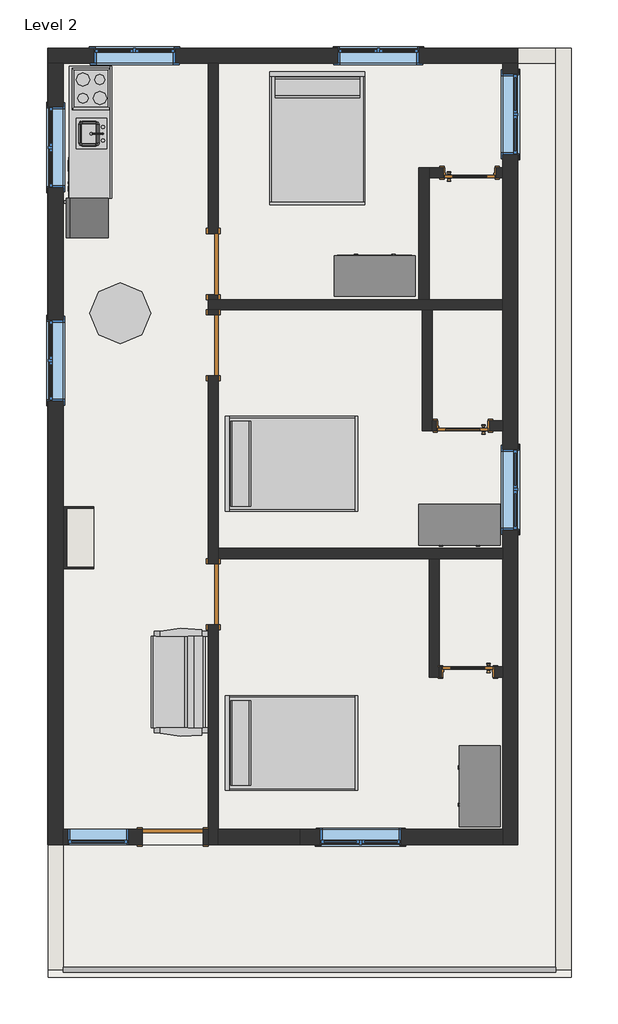
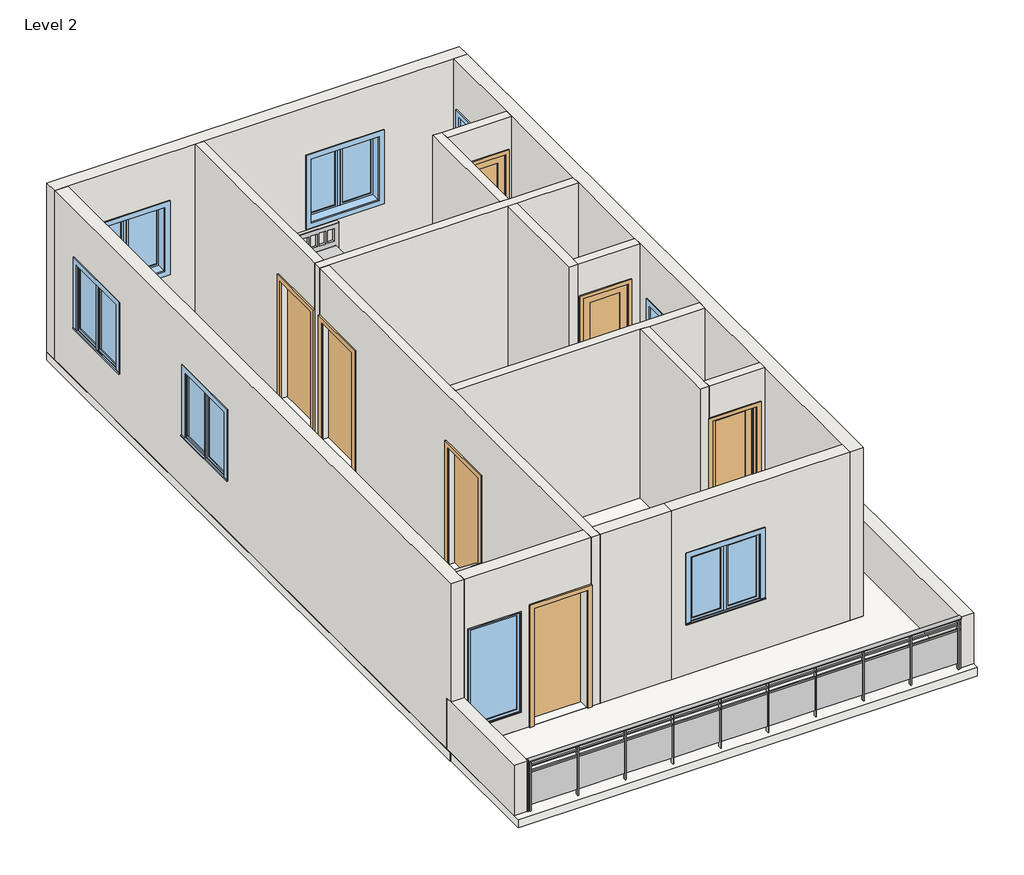
# One storey, incomplete: 20 walls, 9 furniture elements, 8 windows, 7 doors, 4 proxies, 2 slabs, 1 flow terminal, 1 railing.
"""IFC4 building model written with IfcOpenShell, lengths in millimetres."""

from ifc_helpers import new_model, si_unit, point, frame, origin, place, context, project, spatial, polyline, ellipse_curve, trimmed, outline, extrude, faceted_brep, transform, mapped, element, save
from ifc_brep_helpers import plane_surface, extruded_surface, advanced_brep
from components import proxy_a6faaae8, proxy_45b28599, kitchenette_medium_kitchenette_medium_844211aa, proxy_c523a7b7, m_door_interior_single_1_panel_wood_750_x_2400mm_65023cff, m_door_interior_single_1_panel_wood_750_x_2400mm_f8366a1a, door_16372e1c, door_686f89d2, door_0ca8825f, flow_terminal_871c2e40, furniture_096e7f55, furniture_c6510c7c, m_dresser_1220_x_1830_x_0610mm_7cb11019, m_sofa_pensi_2134mm_8f487940, furniture_905aceb5, walls_2_walls_1_3d7729ba, window_534dcd48, window_c796fc87

model = new_model("IFC4")

# Units and contexts
model_context = context("Model", 3, world=origin())
ifc_project = project(units=[si_unit("LENGTHUNIT", "METRE", prefix="MILLI")], contexts=[model_context])

# Site, building, storey
site = spatial("IfcSite", under=ifc_project)
building = spatial("IfcBuilding", under=site)
storey = spatial("IfcBuildingStorey", under=building, Name="Level 2", Elevation=3200.4)

# Proxies
placement = place(None, origin())
proxy_shape = proxy_a6faaae8(model_context)
element("IfcBuildingElementProxy", 1, Name="Cook Top-4 Unit2 : 22\" x 20\"", ObjectType="Cook Top-4 Unit2 : 22\" x 20\"", at=placement, inside=storey, context=model_context, shape_type="MappedRepresentation", body=[
    mapped(proxy_shape, transform((-8891.8371236, 5030.6122215, 3200.4), x_axis=(0.0, -1.0000000000000002, 0.0), y_axis=(1.0000000000000002, 0.0, 0.0), z_axis=(0.0, 0.0, 1.0))),
])
proxy_2_shape = proxy_45b28599(model_context)
element("IfcBuildingElementProxy", 2, Name="Dishwasher : 24\" x 24\" x 34\"", ObjectType="Dishwasher : 24\" x 24\" x 34\"", at=placement, inside=storey, context=model_context, shape_type="MappedRepresentation", body=[
    mapped(proxy_2_shape, transform((-9183.6866883, 4079.42969, 3200.4), x_axis=(0.0, -1.0000000000000002, 0.0), y_axis=(1.0000000000000002, 0.0, 0.0), z_axis=(0.0, 0.0, 1.0))),
])
kitchenette_medium_kitchenette_medium_shape = kitchenette_medium_kitchenette_medium_844211aa(model_context)
element("IfcBuildingElementProxy", 3, Name="Kitchenette - Medium : Kitchenette - Medium", ObjectType="Kitchenette - Medium : Kitchenette - Medium", at=placement, inside=storey, context=model_context, shape_type="MappedRepresentation", body=[
    mapped(kitchenette_medium_kitchenette_medium_shape, transform((-8587.0371236, 4706.4499264, 3200.4), x_axis=(0.0, -1.0000000000000002, 0.0), y_axis=(1.0000000000000002, 0.0, 0.0), z_axis=(0.0, 0.0, 1.0))),
])
proxy_3_shape = proxy_c523a7b7(model_context)
element("IfcBuildingElementProxy", 4, Name="Refrigerator : 24\" x 25\" LH", ObjectType="Refrigerator : 24\" x 25\" LH", at=placement, inside=storey, context=model_context, shape_type="MappedRepresentation", body=[
    mapped(proxy_3_shape, transform((-8937.486095, 3093.8622215, 3200.4), x_axis=(0.0, -1.0000000000000002, 0.0), y_axis=(1.0000000000000002, 0.0, 0.0), z_axis=(0.0, 0.0, 1.0))),
])

# Doors
m_door_interior_single_1_panel_wood_750_x_2400mm_shape = m_door_interior_single_1_panel_wood_750_x_2400mm_65023cff(model_context)
element("IfcDoor", 5, ObjectType="M_Door-Interior-Single-1_Panel-Wood : 750 x 2400mm", at=placement, inside=storey, context=model_context, shape_type="MappedRepresentation", body=[
    mapped(m_door_interior_single_1_panel_wood_750_x_2400mm_shape, transform((-3214.9371236, 3770.1372215, 3200.4), x_axis=(1.0, 0.0, 0.0), y_axis=(0.0, 1.0, 0.0), z_axis=(0.0, 0.0, 1.0))),
])
element("IfcDoor", 6, ObjectType="M_Door-Interior-Single-1_Panel-Wood : 750 x 2400mm", at=placement, inside=storey, context=model_context, shape_type="MappedRepresentation", body=[
    mapped(m_door_interior_single_1_panel_wood_750_x_2400mm_shape, transform((-3240.3371236, -3716.5127785, 3200.4), x_axis=(-1.0, 0.0, 0.0), y_axis=(0.0, -1.0, 0.0), z_axis=(0.0, 0.0, 1.0))),
])
m_door_interior_single_1_panel_wood_750_x_2400mm_2_shape = m_door_interior_single_1_panel_wood_750_x_2400mm_f8366a1a(model_context)
element("IfcDoor", 7, ObjectType="M_Door-Interior-Single-1_Panel-Wood : 750 x 2400mm", at=placement, inside=storey, context=model_context, shape_type="MappedRepresentation", body=[
    mapped(m_door_interior_single_1_panel_wood_750_x_2400mm_2_shape, transform((-3317.235433, -27.8011227, 3200.4), x_axis=(-1.0, 0.0, 0.0), y_axis=(0.0, -1.0, 0.0), z_axis=(0.0, 0.0, 1.0))),
])
door_shape = door_16372e1c(model_context)
element("IfcDoor", 8, ObjectType="Single-Flush : 36\" x 84\"", at=placement, inside=storey, context=model_context, shape_type="MappedRepresentation", body=[
    mapped(door_shape, transform((-7063.0371236, 2401.7122215, 3200.4), x_axis=(0.0, -1.0, 0.0), y_axis=(1.0, 0.0, 0.0), z_axis=(0.0, 0.0, 1.0))),
])
door_2_shape = door_686f89d2(model_context)
element("IfcDoor", 9, ObjectType="Single-Flush : 36\" x 84\"", at=placement, inside=storey, context=model_context, shape_type="MappedRepresentation", body=[
    mapped(door_2_shape, transform((-7063.0371236, 1182.5122215, 3200.4), x_axis=(0.0, 1.0, 0.0), y_axis=(-1.0, 0.0, 0.0), z_axis=(0.0, 0.0, 1.0))),
])
element("IfcDoor", 10, ObjectType="Single-Flush : 36\" x 84\"", at=placement, inside=storey, context=model_context, shape_type="MappedRepresentation", body=[
    mapped(door_2_shape, transform((-7063.0371236, -2551.2877785, 3200.4), x_axis=(0.0, 1.0, 0.0), y_axis=(-1.0, 0.0, 0.0), z_axis=(0.0, 0.0, 1.0))),
])
door_3_shape = door_0ca8825f(model_context)
element("IfcDoor", 11, ObjectType="Single-Flush : 36\" x 84\"", at=placement, inside=storey, context=model_context, shape_type="MappedRepresentation", body=[
    mapped(door_3_shape, transform((-7672.6371236, -6196.1877785, 3200.4), x_axis=(1.0, 0.0, 0.0), y_axis=(0.0, 1.0, 0.0), z_axis=(0.0, 0.0, 1.0))),
])

# Flow terminal
flow_terminal_shape = flow_terminal_871c2e40(model_context)
element("IfcFlowTerminal", 12, ObjectType="Sink Kitchen-Island : 18\" x 18\"", at=placement, inside=storey, context=model_context, shape_type="MappedRepresentation", body=[
    mapped(flow_terminal_shape, transform((-8894.1825247, 4373.2014621, 3186.0), x_axis=(0.0, -1.0000000000000002, 0.0), y_axis=(1.0000000000000002, 0.0, 0.0), z_axis=(0.0, 0.0, 1.0))),
])

# Furniture
furniture_shape = furniture_096e7f55(model_context)
element("IfcFurniture", 13, ObjectType="Bed-Shaker : Double 56\" x 78\"", at=placement, inside=storey, context=model_context, shape_type="MappedRepresentation", body=[
    mapped(furniture_shape, transform((-5481.8871236, 5271.9122215, 3200.4), x_axis=(1.0, 0.0, 0.0), y_axis=(0.0, 1.0, 0.0), z_axis=(0.0, 0.0, 1.0))),
])
element("IfcFurniture", 14, ObjectType="Bed-Shaker : Double 56\" x 78\"", at=placement, inside=storey, context=model_context, shape_type="MappedRepresentation", body=[
    mapped(furniture_shape, transform((-6872.5371236, -576.4377785, 3200.4), x_axis=(0.0, 1.0000000000000004, 0.0), y_axis=(-1.0000000000000004, 0.0, 0.0), z_axis=(0.0, 0.0, 1.0))),
])
element("IfcFurniture", 15, ObjectType="Bed-Shaker : Double 56\" x 78\"", at=placement, inside=storey, context=model_context, shape_type="MappedRepresentation", body=[
    mapped(furniture_shape, transform((-6872.5371236, -4767.4377785, 3200.4), x_axis=(0.0, 1.0, 0.0), y_axis=(-1.0, 0.0, 0.0), z_axis=(0.0, 0.0, 1.0))),
])
furniture_2_shape = furniture_c6510c7c(model_context)
element("IfcFurniture", 16, ObjectType="Counter Top w Sink Hole : 24\" Depth", at=placement, inside=storey, context=model_context, shape_type="MappedRepresentation", body=[
    mapped(furniture_2_shape, transform((-8587.0371236, 4173.0499264, 3186.0), x_axis=(0.0, -1.0000000000000002, 0.0), y_axis=(1.0000000000000002, 0.0, 0.0), z_axis=(0.0, 0.0, 1.0))),
])
m_dresser_1220_x_1830_x_0610mm_shape = m_dresser_1220_x_1830_x_0610mm_7cb11019(model_context)
element("IfcFurniture", 17, ObjectType="M_Dresser : 1220 x 1830 x 0610mm", at=placement, inside=storey, context=model_context, shape_type="MappedRepresentation", body=[
    mapped(m_dresser_1220_x_1830_x_0610mm_shape, transform((-3097.9438637, -1147.1248244, 3200.4), x_axis=(1.0000000000000009, 0.0, 0.0), y_axis=(0.0, 1.0000000000000009, 0.0), z_axis=(0.0, 0.0, 1.0))),
])
element("IfcFurniture", 18, ObjectType="M_Dresser : 1220 x 1830 x 0610mm", at=placement, inside=storey, context=model_context, shape_type="MappedRepresentation", body=[
    mapped(m_dresser_1220_x_1830_x_0610mm_shape, transform((-4909.1553148, 1860.9492674, 3200.4), x_axis=(-1.0000000000000009, 0.0, 0.0), y_axis=(0.0, -1.0000000000000009, 0.0), z_axis=(0.0, 0.0, 1.0))),
])
element("IfcFurniture", 19, ObjectType="M_Dresser : 1220 x 1830 x 0610mm", at=placement, inside=storey, context=model_context, shape_type="MappedRepresentation", body=[
    mapped(m_dresser_1220_x_1830_x_0610mm_shape, transform((-2699.5741695, -5702.9810383, 3200.4), x_axis=(0.0, -1.0, 0.0), y_axis=(1.0, 0.0, 0.0), z_axis=(0.0, 0.0, 1.0))),
])
m_sofa_pensi_2134mm_shape = m_sofa_pensi_2134mm_8f487940(model_context)
element("IfcFurniture", 20, ObjectType="M_Sofa-Pensi : 2134mm", at=placement, inside=storey, context=model_context, shape_type="MappedRepresentation", body=[
    mapped(m_sofa_pensi_2134mm_shape, transform((-7848.1469596, -3593.4815285, 3200.4), x_axis=(0.0, -1.0000000000000002, 0.0), y_axis=(1.0000000000000002, 0.0, 0.0), z_axis=(0.0, 0.0, 1.0))),
])
furniture_3_shape = furniture_905aceb5(model_context)
element("IfcFurniture", 21, ObjectType="Table-Dining Round w Chairs : 36\" Diameter", at=placement, inside=storey, context=model_context, shape_type="MappedRepresentation", body=[
    mapped(furniture_3_shape, transform((-8563.7190908, 1849.99091, 3200.4), x_axis=(1.0, 0.0, 0.0), y_axis=(0.0, 1.0, 0.0), z_axis=(0.0, 0.0, 1.0))),
])

# Railing
element("IfcRailing", 22, ObjectType="Glass Panel - Bottom Fill", at=placement, inside=storey, context=model_context, shape_type="SolidModel", body=[
    advanced_brep(
    [(-9310.9371236, -8151.9877785, 4114.8), (-9310.9371236, -8228.1877785, 4114.8), (-1919.5371236, -8151.9877785, 4114.8), (-1919.5371236, -8228.1877785, 4114.8)],
    [
        (0, 1, ellipse_curve(frame((-9310.9371236, -8190.0877785, 4114.8), z_axis=(-1.0, 0.0, 0.0), x_axis=(0.0, -1.0, 0.0)), 38.1, 28.575)),
        (1, 0, ellipse_curve(frame((-9310.9371236, -8190.0877785, 4114.8), z_axis=(-1.0, 0.0, 0.0), x_axis=(0.0, -1.0, 0.0)), 38.1, 28.575)),
        (2, 3, ellipse_curve(frame((-1919.5371236, -8190.0877785, 4114.8), z_axis=(1.0, 0.0, 0.0), x_axis=(0.0, -1.0, 0.0)), 38.1, 28.575)),
        (3, 2, ellipse_curve(frame((-1919.5371236, -8190.0877785, 4114.8), z_axis=(1.0, 0.0, 0.0), x_axis=(0.0, -1.0, 0.0)), 38.1, 28.575)),
        (0, 2),
        (3, 1),
    ],
    [
        plane_surface(frame((-9310.9371236, -8190.0877785, 4114.8), z_axis=(-1.0, 0.0, 0.0), x_axis=(0.0, 1.0, 0.0))),
        plane_surface(frame((-1919.5371236, -8190.0877785, 4114.8), z_axis=(1.0, 0.0, 0.0), x_axis=(0.0, 1.0, 0.0))),
        extruded_surface(trimmed(ellipse_curve(frame((-1919.5371236, -8190.0877785, 4114.8), z_axis=(-1.0, 0.0, 0.0), x_axis=(0.0, -1.0, 0.0)), 38.1, 28.575), [point((-1919.5371236, -8151.9877785, 4114.8))], [point((-1919.5371236, -8228.1877785, 4114.8))], True, "CARTESIAN"), (-7391.400000000001, 0.0, 0.0), 7391.400000000001),
        extruded_surface(trimmed(ellipse_curve(frame((-1919.5371236, -8190.0877785, 4114.8), z_axis=(-1.0, 0.0, 0.0), x_axis=(0.0, -1.0, 0.0)), 38.1, 28.575), [point((-1919.5371236, -8228.1877785, 4114.8))], [point((-1919.5371236, -8151.9877785, 4114.8))], True, "CARTESIAN"), (-7391.400000000001, 0.0, 0.0), 7391.400000000001),
    ],
    [
        (0, [[1, 2]]),
        (1, [[3, 4]]),
        (2, [[-1, 5, -4, 6]]),
        (3, [[-2, -6, -3, -5]]),
    ],
),
    extrude(outline(polyline([(-9310.9371236, -8202.7877785), (-9310.9371236, -8177.3877785), (-1919.5371236, -8177.3877785), (-1919.5371236, -8202.7877785), (-9310.9371236, -8202.7877785)])), frame((0.0, 0.0, 4000.5), z_axis=(0.0, 0.0, 1.0), x_axis=(1.0, 0.0, 0.0)), (0.0, 0.0, 1.0), 25.4),
    extrude(outline(polyline([(-9310.9371236, -8202.7877785), (-9310.9371236, -8177.3877785), (-1919.5371236, -8177.3877785), (-1919.5371236, -8202.7877785), (-9310.9371236, -8202.7877785)])), frame((0.0, 0.0, 3898.9), z_axis=(0.0, 0.0, 1.0), x_axis=(1.0, 0.0, 0.0)), (0.0, 0.0, 1.0), 25.4),
    extrude(outline(polyline([(-1963.9871236, -8215.4877785), (-1963.9871236, -8164.6877785), (-1951.2871236, -8164.6877785), (-1951.2871236, -8215.4877785), (-1963.9871236, -8215.4877785)])), frame((0.0, 0.0, 3200.4), z_axis=(0.0, 0.0, 1.0), x_axis=(1.0, 0.0, 0.0)), (0.0, 0.0, 1.0), 885.6788223),
    extrude(outline(polyline([(-2770.4371236, -8183.5526215), (-1957.6371236, -8183.5526215), (-1957.6371236, -8189.9026215), (-2770.4371236, -8189.9026215), (-2770.4371236, -8183.5526215)])), frame((0.0, 0.0, 3302.0), z_axis=(0.0, 0.0, 1.0), x_axis=(1.0, 0.0, 0.0)), (0.0, 0.0, 1.0), 596.9),
    extrude(outline(polyline([(-2776.7871236, -8215.4877785), (-2776.7871236, -8164.6877785), (-2764.0871236, -8164.6877785), (-2764.0871236, -8215.4877785), (-2776.7871236, -8215.4877785)])), frame((0.0, 0.0, 3200.4), z_axis=(0.0, 0.0, 1.0), x_axis=(1.0, 0.0, 0.0)), (0.0, 0.0, 1.0), 885.6788223),
    extrude(outline(polyline([(-3583.2371236, -8183.5526215), (-2770.4371236, -8183.5526215), (-2770.4371236, -8189.9026215), (-3583.2371236, -8189.9026215), (-3583.2371236, -8183.5526215)])), frame((0.0, 0.0, 3302.0), z_axis=(0.0, 0.0, 1.0), x_axis=(1.0, 0.0, 0.0)), (0.0, 0.0, 1.0), 596.9),
    extrude(outline(polyline([(-3589.5871236, -8215.4877785), (-3589.5871236, -8164.6877785), (-3576.8871236, -8164.6877785), (-3576.8871236, -8215.4877785), (-3589.5871236, -8215.4877785)])), frame((0.0, 0.0, 3200.4), z_axis=(0.0, 0.0, 1.0), x_axis=(1.0, 0.0, 0.0)), (0.0, 0.0, 1.0), 885.6788223),
    extrude(outline(polyline([(-4396.0371236, -8183.5526215), (-3583.2371236, -8183.5526215), (-3583.2371236, -8189.9026215), (-4396.0371236, -8189.9026215), (-4396.0371236, -8183.5526215)])), frame((0.0, 0.0, 3302.0), z_axis=(0.0, 0.0, 1.0), x_axis=(1.0, 0.0, 0.0)), (0.0, 0.0, 1.0), 596.9),
    extrude(outline(polyline([(-4402.3871236, -8215.4877785), (-4402.3871236, -8164.6877785), (-4389.6871236, -8164.6877785), (-4389.6871236, -8215.4877785), (-4402.3871236, -8215.4877785)])), frame((0.0, 0.0, 3200.4), z_axis=(0.0, 0.0, 1.0), x_axis=(1.0, 0.0, 0.0)), (0.0, 0.0, 1.0), 885.6788223),
    extrude(outline(polyline([(-5208.8371236, -8183.5526215), (-4396.0371236, -8183.5526215), (-4396.0371236, -8189.9026215), (-5208.8371236, -8189.9026215), (-5208.8371236, -8183.5526215)])), frame((0.0, 0.0, 3302.0), z_axis=(0.0, 0.0, 1.0), x_axis=(1.0, 0.0, 0.0)), (0.0, 0.0, 1.0), 596.9),
    extrude(outline(polyline([(-5215.1871236, -8215.4877785), (-5215.1871236, -8164.6877785), (-5202.4871236, -8164.6877785), (-5202.4871236, -8215.4877785), (-5215.1871236, -8215.4877785)])), frame((0.0, 0.0, 3200.4), z_axis=(0.0, 0.0, 1.0), x_axis=(1.0, 0.0, 0.0)), (0.0, 0.0, 1.0), 885.6788223),
    extrude(outline(polyline([(-6021.6371236, -8183.5526215), (-5208.8371236, -8183.5526215), (-5208.8371236, -8189.9026215), (-6021.6371236, -8189.9026215), (-6021.6371236, -8183.5526215)])), frame((0.0, 0.0, 3302.0), z_axis=(0.0, 0.0, 1.0), x_axis=(1.0, 0.0, 0.0)), (0.0, 0.0, 1.0), 596.9),
    extrude(outline(polyline([(-6027.9871236, -8215.4877785), (-6027.9871236, -8164.6877785), (-6015.2871236, -8164.6877785), (-6015.2871236, -8215.4877785), (-6027.9871236, -8215.4877785)])), frame((0.0, 0.0, 3200.4), z_axis=(0.0, 0.0, 1.0), x_axis=(1.0, 0.0, 0.0)), (0.0, 0.0, 1.0), 885.6788223),
    extrude(outline(polyline([(-6834.4371236, -8183.5526215), (-6021.6371236, -8183.5526215), (-6021.6371236, -8189.9026215), (-6834.4371236, -8189.9026215), (-6834.4371236, -8183.5526215)])), frame((0.0, 0.0, 3302.0), z_axis=(0.0, 0.0, 1.0), x_axis=(1.0, 0.0, 0.0)), (0.0, 0.0, 1.0), 596.9),
    extrude(outline(polyline([(-6840.7871236, -8215.4877785), (-6840.7871236, -8164.6877785), (-6828.0871236, -8164.6877785), (-6828.0871236, -8215.4877785), (-6840.7871236, -8215.4877785)])), frame((0.0, 0.0, 3200.4), z_axis=(0.0, 0.0, 1.0), x_axis=(1.0, 0.0, 0.0)), (0.0, 0.0, 1.0), 885.6788223),
    extrude(outline(polyline([(-7647.2371236, -8183.5526215), (-6834.4371236, -8183.5526215), (-6834.4371236, -8189.9026215), (-7647.2371236, -8189.9026215), (-7647.2371236, -8183.5526215)])), frame((0.0, 0.0, 3302.0), z_axis=(0.0, 0.0, 1.0), x_axis=(1.0, 0.0, 0.0)), (0.0, 0.0, 1.0), 596.9),
    extrude(outline(polyline([(-7653.5871236, -8215.4877785), (-7653.5871236, -8164.6877785), (-7640.8871236, -8164.6877785), (-7640.8871236, -8215.4877785), (-7653.5871236, -8215.4877785)])), frame((0.0, 0.0, 3200.4), z_axis=(0.0, 0.0, 1.0), x_axis=(1.0, 0.0, 0.0)), (0.0, 0.0, 1.0), 885.6788223),
    extrude(outline(polyline([(-8460.0371236, -8183.5526215), (-7647.2371236, -8183.5526215), (-7647.2371236, -8189.9026215), (-8460.0371236, -8189.9026215), (-8460.0371236, -8183.5526215)])), frame((0.0, 0.0, 3302.0), z_axis=(0.0, 0.0, 1.0), x_axis=(1.0, 0.0, 0.0)), (0.0, 0.0, 1.0), 596.9),
    extrude(outline(polyline([(-8466.3871236, -8215.4877785), (-8466.3871236, -8164.6877785), (-8453.6871236, -8164.6877785), (-8453.6871236, -8215.4877785), (-8466.3871236, -8215.4877785)])), frame((0.0, 0.0, 3200.4), z_axis=(0.0, 0.0, 1.0), x_axis=(1.0, 0.0, 0.0)), (0.0, 0.0, 1.0), 885.6788223),
    extrude(outline(polyline([(-9272.8371236, -8183.5526215), (-8460.0371236, -8183.5526215), (-8460.0371236, -8189.9026215), (-9272.8371236, -8189.9026215), (-9272.8371236, -8183.5526215)])), frame((0.0, 0.0, 3302.0), z_axis=(0.0, 0.0, 1.0), x_axis=(1.0, 0.0, 0.0)), (0.0, 0.0, 1.0), 596.9),
    extrude(outline(polyline([(-9279.1871236, -8215.4877785), (-9279.1871236, -8164.6877785), (-9266.4871236, -8164.6877785), (-9266.4871236, -8215.4877785), (-9279.1871236, -8215.4877785)])), frame((0.0, 0.0, 3200.4), z_axis=(0.0, 0.0, 1.0), x_axis=(1.0, 0.0, 0.0)), (0.0, 0.0, 1.0), 885.6788223),
    extrude(outline(polyline([(-1932.2371236, -8199.6127785), (-1932.2371236, -8180.5627785), (-1913.1871236, -8180.5627785), (-1913.1871236, -8199.6127785), (-1932.2371236, -8199.6127785)])), frame((0.0, 0.0, 3200.4), z_axis=(0.0, 0.0, 1.0), x_axis=(1.0, 0.0, 0.0)), (0.0, 0.0, 1.0), 885.6788223),
    extrude(outline(polyline([(-9317.2871236, -8199.6127785), (-9317.2871236, -8180.5627785), (-9298.2371236, -8180.5627785), (-9298.2371236, -8199.6127785), (-9317.2871236, -8199.6127785)])), frame((0.0, 0.0, 3200.4), z_axis=(0.0, 0.0, 1.0), x_axis=(1.0, 0.0, 0.0)), (0.0, 0.0, 1.0), 885.6788223),
])

# Slabs
element("IfcSlab", 23, ObjectType="6\"", at=placement, inside=storey, context=model_context, shape_type="SweptSolid", body=[
    extrude(outline(polyline([(-2491.0371236, 5640.2122215), (-2491.0371236, -6310.4877785), (-9544.743556, -6310.4877785), (-9544.743556, 5640.2122215), (-2491.0371236, 5640.2122215)])), frame((0.0, 0.0, 3048.0), z_axis=(0.0, 0.0, 1.0), x_axis=(1.0, 0.0, 0.0)), (0.0, 0.0, 1.0), 152.4),
])
element("IfcSlab", 24, ObjectType="6\"", at=placement, inside=storey, context=model_context, shape_type="SweptSolid", body=[
    extrude(outline(polyline([(-1690.9371236, 5640.2122215), (-1690.9371236, -8304.3877785), (-9538.393556, -8304.3877785), (-9538.393556, 5640.2122215), (-1690.9371236, 5640.2122215)])), frame((0.0, 0.0, 3048.0), z_axis=(0.0, 0.0, 1.0), x_axis=(1.0, 0.0, 0.0)), (0.0, 0.0, 1.0), 152.4),
])

# Walls
element("IfcWall", 25, ObjectType="6\"", at=placement, inside=storey, context=model_context, shape_type="Brep", body=[
    faceted_brep([(-2719.6371236, 1868.3122215, 3200.4), (-3824.5371236, 1868.3122215, 3200.4), (-3976.9371236, 1868.3122215, 3200.4), (-6986.8371236, 1868.3122215, 3200.4), (-7139.2371236, 1868.3122215, 3200.4), (-7139.2371236, 1868.3122215, 6248.4), (-6986.8371236, 1868.3122215, 6248.4), (-3976.9371236, 1868.3122215, 6248.4), (-3824.5371236, 1868.3122215, 6248.4), (-2719.6371236, 1868.3122215, 6248.4), (-2719.6371236, 1715.9122215, 3200.4), (-2719.6371236, 1715.9122215, 6248.4), (-3774.435433, 1715.9122215, 6248.4), (-3926.835433, 1715.9122215, 6248.4), (-6986.8371236, 1715.9122215, 6248.4), (-7139.2371236, 1715.9122215, 6248.4), (-7139.2371236, 1715.9122215, 3200.4), (-6986.8371236, 1715.9122215, 3200.4), (-3926.835433, 1715.9122215, 3200.4), (-3774.435433, 1715.9122215, 3200.4)], [[[0, 1, 2, 3, 4, 5, 6, 7, 8, 9]], [[10, 11, 12, 13, 14, 15, 16, 17, 18, 19]], [[4, 3, 2, 1, 0, 10, 19, 18, 17, 16]], [[9, 8, 7, 6, 5, 15, 14, 13, 12, 11]], [[0, 9, 11, 10]], [[5, 4, 16, 15]]]),
])
element("IfcWall", 26, ObjectType="6\"", at=placement, inside=storey, context=model_context, shape_type="SweptSolid", body=[
    extrude(outline(polyline([(1944.5122215, 5334.0), (1944.5122215, 3200.4), (1868.3122215, 3200.4), (1868.3122215, 6248.4), (5411.6122215, 6248.4), (5411.6122215, 3200.4), (2858.9122215, 3200.4), (2858.9122215, 5334.0), (1944.5122215, 5334.0)])), frame((-7139.2371236, 0.0, 0.0), z_axis=(1.0, 0.0, 0.0), x_axis=(0.0, 1.0, 0.0)), (0.0, 0.0, 1.0), 152.4),
])
element("IfcWall", 27, ObjectType="6\"", at=placement, inside=storey, context=model_context, shape_type="Brep", body=[
    faceted_brep([(-3824.5371236, 1868.3122215, 3200.4), (-3824.5371236, 3697.1122215, 3200.4), (-3824.5371236, 3849.5122215, 3200.4), (-3824.5371236, 3849.5122215, 6248.4), (-3824.5371236, 3697.1122215, 6248.4), (-3824.5371236, 1868.3122215, 6248.4), (-3976.9371236, 1868.3122215, 3200.4), (-3976.9371236, 1868.3122215, 6248.4), (-3976.9371236, 3849.5122215, 6248.4), (-3976.9371236, 3849.5122215, 3200.4)], [[[0, 1, 2, 3, 4, 5]], [[6, 7, 8, 9]], [[2, 1, 0, 6, 9]], [[5, 4, 3, 8, 7]], [[0, 5, 7, 6]], [[3, 2, 9, 8]]]),
])
element("IfcWall", 28, ObjectType="6\"", at=placement, inside=storey, context=model_context, shape_type="SweptSolid", body=[
    extrude(outline(polyline([(6248.4, -2719.6371236), (6248.4, -3824.5371236), (3200.4, -3824.5371236), (3200.4, -3614.9371236), (5625.4, -3614.9371236), (5625.4, -2814.9371236), (3200.4, -2814.9371236), (3200.4, -2719.6371236), (6248.4, -2719.6371236)])), frame((0.0, 3697.1122215, 0.0), z_axis=(0.0, 1.0, 0.0), x_axis=(0.0, 0.0, 1.0)), (0.0, 0.0, 1.0), 152.4),
])
element("IfcWall", 29, ObjectType="6\"", at=placement, inside=storey, context=model_context, shape_type="Brep", body=[
    faceted_brep([(-2719.6371236, -1865.4877785, 3200.4), (-6986.8371236, -1865.4877785, 3200.4), (-6986.8371236, -1865.4877785, 6248.4), (-2719.6371236, -1865.4877785, 6248.4), (-2719.6371236, -2017.8877785, 3200.4), (-2719.6371236, -2017.8877785, 6248.4), (-3672.1371236, -2017.8877785, 6248.4), (-3824.5371236, -2017.8877785, 6248.4), (-6986.8371236, -2017.8877785, 6248.4), (-6986.8371236, -2017.8877785, 3200.4), (-3824.5371236, -2017.8877785, 3200.4), (-3672.1371236, -2017.8877785, 3200.4)], [[[0, 1, 2, 3]], [[4, 5, 6, 7, 8, 9, 10, 11]], [[1, 0, 4, 11, 10, 9]], [[3, 2, 8, 7, 6, 5]], [[0, 3, 5, 4]], [[2, 1, 9, 8]]]),
])
element("IfcWall", 30, ObjectType="6\"", at=placement, inside=storey, context=model_context, shape_type="Brep", body=[
    faceted_brep([(-7139.2371236, 725.3122215, 3200.4), (-7139.2371236, -2094.0877785, 3200.4), (-7139.2371236, -2094.0877785, 5334.0), (-7139.2371236, -3008.4877785, 5334.0), (-7139.2371236, -3008.4877785, 3200.4), (-7139.2371236, -6081.8877785, 3200.4), (-7139.2371236, -6310.4877785, 3200.4), (-7139.2371236, -6310.4877785, 6248.4), (-7139.2371236, -6081.8877785, 6248.4), (-7139.2371236, 1715.9122215, 6248.4), (-7139.2371236, 1715.9122215, 3200.4), (-7139.2371236, 1639.7122215, 3200.4), (-7139.2371236, 1639.7122215, 5334.0), (-7139.2371236, 725.3122215, 5334.0), (-6986.8371236, -2094.0877785, 5334.0), (-6986.8371236, -2094.0877785, 3200.4), (-6986.8371236, -2017.8877785, 3200.4), (-6986.8371236, -1865.4877785, 3200.4), (-6986.8371236, 725.3122215, 3200.4), (-6986.8371236, 725.3122215, 5334.0), (-6986.8371236, 1639.7122215, 5334.0), (-6986.8371236, 1639.7122215, 3200.4), (-6986.8371236, 1715.9122215, 3200.4), (-6986.8371236, 1715.9122215, 6248.4), (-6986.8371236, -1865.4877785, 6248.4), (-6986.8371236, -2017.8877785, 6248.4), (-6986.8371236, -6081.8877785, 6248.4), (-6986.8371236, -6310.4877785, 6248.4), (-6986.8371236, -6310.4877785, 3200.4), (-6986.8371236, -6081.8877785, 3200.4), (-6986.8371236, -3008.4877785, 3200.4), (-6986.8371236, -3008.4877785, 5334.0)], [[[0, 1, 2, 3, 4, 5, 6, 7, 8, 9, 10, 11, 12, 13]], [[14, 15, 16, 17, 18, 19, 20, 21, 22, 23, 24, 25, 26, 27, 28, 29, 30, 31]], [[22, 21, 11, 10]], [[30, 29, 28, 6, 5, 4]], [[18, 17, 16, 15, 1, 0]], [[9, 8, 7, 27, 26, 25, 24, 23]], [[10, 9, 23, 22]], [[7, 6, 28, 27]], [[12, 11, 21, 20]], [[13, 12, 20, 19]], [[0, 13, 19, 18]], [[2, 1, 15, 14]], [[3, 2, 14, 31]], [[4, 3, 31, 30]]]),
])
element("IfcWall", 31, ObjectType="6\"", at=placement, inside=storey, context=model_context, shape_type="Brep", body=[
    faceted_brep([(-3824.5371236, -2017.8877785, 3200.4), (-3824.5371236, -3795.8877785, 3200.4), (-3824.5371236, -3795.8877785, 6248.4), (-3824.5371236, -2017.8877785, 6248.4), (-3672.1371236, -2017.8877785, 3200.4), (-3672.1371236, -2017.8877785, 6248.4), (-3672.1371236, -3643.4877785, 6248.4), (-3672.1371236, -3795.8877785, 6248.4), (-3672.1371236, -3795.8877785, 3200.4), (-3672.1371236, -3643.4877785, 3200.4)], [[[0, 1, 2, 3]], [[4, 5, 6, 7, 8, 9]], [[1, 0, 4, 9, 8]], [[3, 2, 7, 6, 5]], [[0, 3, 5, 4]], [[2, 1, 8, 7]]]),
])
element("IfcWall", 32, ObjectType="6\"", at=placement, inside=storey, context=model_context, shape_type="SweptSolid", body=[
    extrude(outline(polyline([(6248.4, -2719.6371236), (6248.4, -3672.1371236), (3200.4, -3672.1371236), (3200.4, -3640.3371236), (5625.4, -3640.3371236), (5625.4, -2840.3371236), (3200.4, -2840.3371236), (3200.4, -2719.6371236), (6248.4, -2719.6371236)])), frame((0.0, -3795.8877785, 0.0), z_axis=(0.0, 1.0, 0.0), x_axis=(0.0, 0.0, 1.0)), (0.0, 0.0, 1.0), 152.4),
])
element("IfcWall", 33, ObjectType="6\"", at=placement, inside=storey, context=model_context, shape_type="Brep", body=[
    faceted_brep([(-3926.835433, 1715.9122215, 3200.4), (-3926.835433, -100.8261227, 3200.4), (-3926.835433, -100.8261227, 6248.4), (-3926.835433, 1715.9122215, 6248.4), (-3774.435433, 1715.9122215, 3200.4), (-3774.435433, 1715.9122215, 6248.4), (-3774.435433, 51.5738773, 6248.4), (-3774.435433, -100.8261227, 6248.4), (-3774.435433, -100.8261227, 3200.4), (-3774.435433, 51.5738773, 3200.4)], [[[0, 1, 2, 3]], [[4, 5, 6, 7, 8, 9]], [[1, 0, 4, 9, 8]], [[3, 2, 7, 6, 5]], [[2, 1, 8, 7]], [[0, 3, 5, 4]]]),
])
element("IfcWall", 34, ObjectType="6\"", at=placement, inside=storey, context=model_context, shape_type="SweptSolid", body=[
    extrude(outline(polyline([(6248.4, -2719.6371236), (6248.4, -3774.435433), (3200.4, -3774.435433), (3200.4, -3717.235433), (5625.4, -3717.235433), (5625.4, -2917.235433), (3200.4, -2917.235433), (3200.4, -2719.6371236), (6248.4, -2719.6371236)])), frame((0.0, -100.8261227, 0.0), z_axis=(0.0, 1.0, 0.0), x_axis=(0.0, 0.0, 1.0)), (0.0, 0.0, 1.0), 152.4),
])
element("IfcWall", 35, ObjectType="9\"", at=placement, inside=storey, context=model_context, shape_type="Brep", body=[
    faceted_brep([(-9539.5371236, 5411.6122215, 3200.4), (-9310.9371236, 5411.6122215, 3200.4), (-7139.2371236, 5411.6122215, 3200.4), (-6986.8371236, 5411.6122215, 3200.4), (-2719.6371236, 5411.6122215, 3200.4), (-2605.3371236, 5411.6122215, 3200.4), (-2605.3371236, 5411.6122215, 4114.8), (-2491.0371236, 5411.6122215, 4114.8), (-2491.0371236, 5411.6122215, 6248.4), (-2719.6371236, 5411.6122215, 6248.4), (-6986.8371236, 5411.6122215, 6248.4), (-7139.2371236, 5411.6122215, 6248.4), (-9310.9371236, 5411.6122215, 6248.4), (-9539.5371236, 5411.6122215, 6248.4), (-7632.9835233, 5411.6122215, 5334.0), (-7632.9835233, 5411.6122215, 4114.8), (-8852.1835233, 5411.6122215, 4114.8), (-8852.1835233, 5411.6122215, 5334.0), (-3975.3835233, 5411.6122215, 5334.0), (-3975.3835233, 5411.6122215, 4114.8), (-5194.5835233, 5411.6122215, 4114.8), (-5194.5835233, 5411.6122215, 5334.0), (-9539.5371236, 5640.2122215, 3200.4), (-9539.5371236, 5640.2122215, 6248.4), (-2491.0371236, 5640.2122215, 6248.4), (-2491.0371236, 5640.2122215, 4114.8), (-2605.3371236, 5640.2122215, 4114.8), (-2605.3371236, 5640.2122215, 3200.4), (-7632.9835233, 5640.2122215, 5334.0), (-8852.1835233, 5640.2122215, 5334.0), (-8852.1835233, 5640.2122215, 4114.8), (-7632.9835233, 5640.2122215, 4114.8), (-3975.3835233, 5640.2122215, 5334.0), (-5194.5835233, 5640.2122215, 5334.0), (-5194.5835233, 5640.2122215, 4114.8), (-3975.3835233, 5640.2122215, 4114.8)], [[[0, 1, 2, 3, 4, 5, 6, 7, 8, 9, 10, 11, 12, 13], [14, 15, 16, 17], [18, 19, 20, 21]], [[22, 23, 24, 25, 26, 27], [28, 29, 30, 31], [32, 33, 34, 35]], [[5, 4, 3, 2, 1, 0, 22, 27]], [[13, 12, 11, 10, 9, 8, 24, 23]], [[0, 13, 23, 22]], [[6, 5, 27, 26]], [[25, 7, 6, 26]], [[8, 7, 25, 24]], [[15, 14, 28, 31]], [[16, 15, 31, 30]], [[17, 16, 30, 29]], [[14, 17, 29, 28]], [[19, 18, 32, 35]], [[20, 19, 35, 34]], [[21, 20, 34, 33]], [[18, 21, 33, 32]]]),
])
element("IfcWall", 36, ObjectType="9\"", at=placement, inside=storey, context=model_context, shape_type="Brep", body=[
    faceted_brep([(-9310.9371236, -8190.0877785, 3200.4), (-9310.9371236, -6310.4877785, 3200.4), (-9310.9371236, -6196.1877785, 3200.4), (-9310.9371236, -6196.1877785, 4114.8), (-9310.9371236, -6310.4877785, 4114.8), (-9310.9371236, -8190.0877785, 4114.8), (-9539.5371236, -8190.0877785, 3200.4), (-9539.5371236, -8190.0877785, 4114.8), (-9539.5371236, -6310.4877785, 4114.8), (-9539.5371236, -6196.1877785, 4114.8), (-9539.5371236, -6196.1877785, 3200.4)], [[[0, 1, 2, 3, 4, 5]], [[6, 7, 8, 9, 10]], [[2, 1, 0, 6, 10]], [[3, 2, 10, 9]], [[5, 4, 3, 9, 8, 7]], [[0, 5, 7, 6]]]),
])
element("IfcWall", 37, ObjectType="9\"", at=placement, inside=storey, context=model_context, shape_type="Brep", body=[
    faceted_brep([(-1919.5371236, 5640.2122215, 3200.4), (-1919.5371236, 5411.6122215, 3200.4), (-1919.5371236, -8190.0877785, 3200.4), (-1919.5371236, -8190.0877785, 4114.8), (-1919.5371236, 5411.6122215, 4114.8), (-1919.5371236, 5640.2122215, 4114.8), (-1690.9371236, 5640.2122215, 3200.4), (-1690.9371236, 5640.2122215, 4114.8), (-1690.9371236, -8190.0877785, 4114.8), (-1690.9371236, -8190.0877785, 3200.4)], [[[0, 1, 2, 3, 4, 5]], [[6, 7, 8, 9]], [[2, 1, 0, 6, 9]], [[3, 2, 9, 8]], [[5, 4, 3, 8, 7]], [[0, 5, 7, 6]]]),
])
element("IfcWall", 38, ObjectType="9\"", at=placement, inside=storey, context=model_context, shape_type="Brep", body=[
    faceted_brep([(-2719.6371236, 5411.6122215, 6248.4), (-2719.6371236, 5411.6122215, 3200.4), (-2719.6371236, 3849.5122215, 3200.4), (-2719.6371236, 3697.1122215, 3200.4), (-2719.6371236, 1868.3122215, 3200.4), (-2719.6371236, 1715.9122215, 3200.4), (-2719.6371236, 51.5738773, 3200.4), (-2719.6371236, -100.8261227, 3200.4), (-2719.6371236, -1865.4877785, 3200.4), (-2719.6371236, -2017.8877785, 3200.4), (-2719.6371236, -3643.4877785, 3200.4), (-2719.6371236, -3795.8877785, 3200.4), (-2719.6371236, -6081.8877785, 3200.4), (-2719.6371236, -6310.4877785, 3200.4), (-2719.6371236, -6310.4877785, 6248.4), (-2719.6371236, -6081.8877785, 6248.4), (-2719.6371236, -3795.8877785, 6248.4), (-2719.6371236, -3643.4877785, 6248.4), (-2719.6371236, -2017.8877785, 6248.4), (-2719.6371236, -1865.4877785, 6248.4), (-2719.6371236, -100.8261227, 6248.4), (-2719.6371236, 51.5738773, 6248.4), (-2719.6371236, 1715.9122215, 6248.4), (-2719.6371236, 1868.3122215, 6248.4), (-2719.6371236, 3697.1122215, 6248.4), (-2719.6371236, 3849.5122215, 6248.4), (-2719.6371236, 4038.7165003, 5334.0), (-2719.6371236, 4038.7165003, 4114.8), (-2719.6371236, 5257.9165003, 4114.8), (-2719.6371236, 5257.9165003, 5334.0), (-2719.6371236, -1594.0526718, 5334.0), (-2719.6371236, -1594.0526718, 4114.8), (-2719.6371236, -374.8526718, 4114.8), (-2719.6371236, -374.8526718, 5334.0), (-2491.0371236, 5411.6122215, 3200.4), (-2491.0371236, 5411.6122215, 4114.8), (-2491.0371236, 5411.6122215, 6248.4), (-2491.0371236, -6310.4877785, 6248.4), (-2491.0371236, -6310.4877785, 3200.4), (-2491.0371236, 4038.7165003, 5334.0), (-2491.0371236, 5257.9165003, 5334.0), (-2491.0371236, 5257.9165003, 4114.8), (-2491.0371236, 4038.7165003, 4114.8), (-2491.0371236, -1594.0526718, 5334.0), (-2491.0371236, -374.8526718, 5334.0), (-2491.0371236, -374.8526718, 4114.8), (-2491.0371236, -1594.0526718, 4114.8), (-2605.3371236, 5411.6122215, 3200.4)], [[[0, 1, 2, 3, 4, 5, 6, 7, 8, 9, 10, 11, 12, 13, 14, 15, 16, 17, 18, 19, 20, 21, 22, 23, 24, 25], [26, 27, 28, 29], [30, 31, 32, 33]], [[34, 35, 36, 37, 38], [39, 40, 41, 42], [43, 44, 45, 46]], [[13, 12, 11, 10, 9, 8, 7, 6, 5, 4, 3, 2, 1, 47, 34, 38]], [[0, 25, 24, 23, 22, 21, 20, 19, 18, 17, 16, 15, 14, 37, 36]], [[14, 13, 38, 37]], [[0, 36, 35, 34, 47, 1]], [[27, 26, 39, 42]], [[28, 27, 42, 41]], [[29, 28, 41, 40]], [[26, 29, 40, 39]], [[31, 30, 43, 46]], [[32, 31, 46, 45]], [[33, 32, 45, 44]], [[30, 33, 44, 43]]]),
])
element("IfcWall", 39, ObjectType="9\"", at=placement, inside=storey, context=model_context, shape_type="SweptSolid", body=[
    extrude(outline(polyline([(3200.4, -2719.6371236), (6248.4, -2719.6371236), (6248.4, -5767.6371236), (3200.4, -5767.6371236), (3200.4, -2719.6371236)]), holes=[polyline([(5334.0, -5461.2835233), (5334.0, -4242.0835233), (4114.8, -4242.0835233), (4114.8, -5461.2835233), (5334.0, -5461.2835233)])]), frame((0.0, -6310.4877785, 0.0), z_axis=(0.0, 1.0, 0.0), x_axis=(0.0, 0.0, 1.0)), (0.0, 0.0, 1.0), 228.6),
])
element("IfcWall", 40, ObjectType="9\"", at=placement, inside=storey, context=model_context, shape_type="SweptSolid", body=[
    extrude(outline(polyline([(-6986.8371236, -6081.8877785), (-5767.6371236, -6081.8877785), (-5767.6371236, -6310.4877785), (-6986.8371236, -6310.4877785), (-6986.8371236, -6081.8877785)])), frame((0.0, 0.0, 3200.4), z_axis=(0.0, 0.0, 1.0), x_axis=(1.0, 0.0, 0.0)), (0.0, 0.0, 1.0), 3048.0),
])
element("IfcWall", 41, ObjectType="9\"", at=placement, inside=storey, context=model_context, shape_type="Brep", body=[
    faceted_brep([(-7215.4371236, -6310.4877785, 5334.0), (-7215.4371236, -6310.4877785, 3200.4), (-7139.2371236, -6310.4877785, 3200.4), (-7139.2371236, -6310.4877785, 6248.4), (-9310.9371236, -6310.4877785, 6248.4), (-9310.9371236, -6310.4877785, 4114.8), (-9310.9371236, -6310.4877785, 3200.4), (-8129.8371236, -6310.4877785, 3200.4), (-8129.8371236, -6310.4877785, 5334.0), (-9247.4371236, -6310.4877785, 5334.0), (-8333.0371236, -6310.4877785, 5334.0), (-8333.0371236, -6310.4877785, 3505.2), (-9247.4371236, -6310.4877785, 3505.2), (-7139.2371236, -6081.8877785, 3200.4), (-7215.4371236, -6081.8877785, 3200.4), (-7215.4371236, -6081.8877785, 5334.0), (-8129.8371236, -6081.8877785, 5334.0), (-8129.8371236, -6081.8877785, 3200.4), (-9310.9371236, -6081.8877785, 3200.4), (-9310.9371236, -6081.8877785, 6248.4), (-7139.2371236, -6081.8877785, 6248.4), (-9247.4371236, -6081.8877785, 5334.0), (-9247.4371236, -6081.8877785, 3505.2), (-8333.0371236, -6081.8877785, 3505.2), (-8333.0371236, -6081.8877785, 5334.0), (-9310.9371236, -6196.1877785, 3200.4)], [[[0, 1, 2, 3, 4, 5, 6, 7, 8], [9, 10, 11, 12]], [[13, 14, 15, 16, 17, 18, 19, 20], [21, 22, 23, 24]], [[7, 6, 25, 18, 17]], [[2, 1, 14, 13]], [[4, 3, 20, 19]], [[3, 2, 13, 20]], [[4, 19, 18, 25, 6, 5]], [[15, 14, 1, 0]], [[16, 15, 0, 8]], [[17, 16, 8, 7]], [[22, 21, 9, 12]], [[23, 22, 12, 11]], [[24, 23, 11, 10]], [[21, 24, 10, 9]]]),
])
element("IfcWall", 42, ObjectType="9\"", at=placement, inside=storey, context=model_context, shape_type="Brep", body=[
    faceted_brep([(-9310.9371236, -6196.1877785, 3200.4), (-9310.9371236, -6081.8877785, 3200.4), (-9310.9371236, 5411.6122215, 3200.4), (-9310.9371236, 5411.6122215, 6248.4), (-9310.9371236, -6081.8877785, 6248.4), (-9310.9371236, -6310.4877785, 6248.4), (-9310.9371236, -6310.4877785, 4114.8), (-9310.9371236, -6196.1877785, 4114.8), (-9310.9371236, 1562.2165003, 5334.0), (-9310.9371236, 1562.2165003, 4114.8), (-9310.9371236, 343.0165003, 4114.8), (-9310.9371236, 343.0165003, 5334.0), (-9310.9371236, 4762.6165003, 5334.0), (-9310.9371236, 4762.6165003, 4114.8), (-9310.9371236, 3543.4165003, 4114.8), (-9310.9371236, 3543.4165003, 5334.0), (-9539.5371236, -6196.1877785, 3200.4), (-9539.5371236, -6196.1877785, 4114.8), (-9539.5371236, -6310.4877785, 4114.8), (-9539.5371236, -6310.4877785, 6248.4), (-9539.5371236, 5411.6122215, 6248.4), (-9539.5371236, 5411.6122215, 3200.4), (-9539.5371236, 1562.2165003, 5334.0), (-9539.5371236, 343.0165003, 5334.0), (-9539.5371236, 343.0165003, 4114.8), (-9539.5371236, 1562.2165003, 4114.8), (-9539.5371236, 4762.6165003, 5334.0), (-9539.5371236, 3543.4165003, 5334.0), (-9539.5371236, 3543.4165003, 4114.8), (-9539.5371236, 4762.6165003, 4114.8)], [[[0, 1, 2, 3, 4, 5, 6, 7], [8, 9, 10, 11], [12, 13, 14, 15]], [[16, 17, 18, 19, 20, 21], [22, 23, 24, 25], [26, 27, 28, 29]], [[2, 1, 0, 16, 21]], [[5, 4, 3, 20, 19]], [[3, 2, 21, 20]], [[0, 7, 17, 16]], [[6, 18, 17, 7]], [[6, 5, 19, 18]], [[9, 8, 22, 25]], [[10, 9, 25, 24]], [[11, 10, 24, 23]], [[8, 11, 23, 22]], [[13, 12, 26, 29]], [[14, 13, 29, 28]], [[15, 14, 28, 27]], [[12, 15, 27, 26]]]),
])
element("IfcWall", 43, ObjectType="9\"", at=placement, inside=storey, context=model_context, shape_type="Brep", body=[
    faceted_brep([(-2605.3371236, 5411.6122215, 3200.4), (-2491.0371236, 5411.6122215, 3200.4), (-1919.5371236, 5411.6122215, 3200.4), (-1919.5371236, 5411.6122215, 4114.8), (-2491.0371236, 5411.6122215, 4114.8), (-2605.3371236, 5411.6122215, 4114.8), (-2605.3371236, 5640.2122215, 3200.4), (-2605.3371236, 5640.2122215, 4114.8), (-2491.0371236, 5640.2122215, 4114.8), (-1919.5371236, 5640.2122215, 4114.8), (-1919.5371236, 5640.2122215, 3200.4)], [[[0, 1, 2, 3, 4, 5]], [[6, 7, 8, 9, 10]], [[2, 1, 0, 6, 10]], [[5, 4, 3, 9, 8, 7]], [[0, 5, 7, 6]], [[3, 2, 10, 9]]]),
])
walls_2_walls_1_shape = walls_2_walls_1_3d7729ba(model_context)
element("IfcWall", 44, ObjectType="Walls 2 : Walls 1", at=placement, inside=storey, context=model_context, shape_type="MappedRepresentation", body=[
    mapped(walls_2_walls_1_shape, transform((0.0, 0.0, 0.0), x_axis=(1.0, 0.0, 0.0), y_axis=(0.0, 1.0, 0.0), z_axis=(0.0, 0.0, 1.0))),
])

# Windows
window_shape = window_534dcd48(model_context)
element("IfcWindow", 45, ObjectType="Casement Dbl with Trim : 48\" x 48\"", at=placement, inside=storey, context=model_context, shape_type="MappedRepresentation", body=[
    mapped(window_shape, transform((-4851.6835233, -6177.1377785, 3200.4), x_axis=(-1.0, 0.0, 0.0), y_axis=(0.0, -1.0, 0.0), z_axis=(0.0, 0.0, 1.0))),
])
element("IfcWindow", 46, ObjectType="Casement Dbl with Trim : 48\" x 48\"", at=placement, inside=storey, context=model_context, shape_type="MappedRepresentation", body=[
    mapped(window_shape, transform((-2624.3871236, -984.4526718, 3200.4), x_axis=(0.0, -1.0, 0.0), y_axis=(1.0, 0.0, 0.0), z_axis=(0.0, 0.0, 1.0))),
])
element("IfcWindow", 47, ObjectType="Casement Dbl with Trim : 48\" x 48\"", at=placement, inside=storey, context=model_context, shape_type="MappedRepresentation", body=[
    mapped(window_shape, transform((-2624.3871236, 4648.3165003, 3200.4), x_axis=(0.0, -1.0, 0.0), y_axis=(1.0, 0.0, 0.0), z_axis=(0.0, 0.0, 1.0))),
])
element("IfcWindow", 48, ObjectType="Casement Dbl with Trim : 48\" x 48\"", at=placement, inside=storey, context=model_context, shape_type="MappedRepresentation", body=[
    mapped(window_shape, transform((-4584.9835233, 5506.8622215, 3200.4), x_axis=(1.0, 0.0, 0.0), y_axis=(0.0, 1.0, 0.0), z_axis=(0.0, 0.0, 1.0))),
])
element("IfcWindow", 49, ObjectType="Casement Dbl with Trim : 48\" x 48\"", at=placement, inside=storey, context=model_context, shape_type="MappedRepresentation", body=[
    mapped(window_shape, transform((-9406.1871236, 4153.0165003, 3200.4), x_axis=(0.0, 1.0, 0.0), y_axis=(-1.0, 0.0, 0.0), z_axis=(0.0, 0.0, 1.0))),
])
element("IfcWindow", 50, ObjectType="Casement Dbl with Trim : 48\" x 48\"", at=placement, inside=storey, context=model_context, shape_type="MappedRepresentation", body=[
    mapped(window_shape, transform((-8242.5835233, 5506.8622215, 3200.4), x_axis=(1.0, 0.0, 0.0), y_axis=(0.0, 1.0, 0.0), z_axis=(0.0, 0.0, 1.0))),
])
element("IfcWindow", 51, ObjectType="Casement Dbl with Trim : 48\" x 48\"", at=placement, inside=storey, context=model_context, shape_type="MappedRepresentation", body=[
    mapped(window_shape, transform((-9406.1871236, 952.6165003, 3200.4), x_axis=(0.0, 1.0, 0.0), y_axis=(-1.0, 0.0, 0.0), z_axis=(0.0, 0.0, 1.0))),
])
window_2_shape = window_c796fc87(model_context)
element("IfcWindow", 52, ObjectType="Fixed : 36\" x 72\"", at=placement, inside=storey, context=model_context, shape_type="MappedRepresentation", body=[
    mapped(window_2_shape, transform((-8828.3371236, -6196.1877785, 3200.4), x_axis=(-1.0, 0.0, 0.0), y_axis=(0.0, -1.0, 0.0), z_axis=(0.0, 0.0, 1.0))),
])

save(model, "model.ifc")

# Revit data of these elements
# Type "Cook Top-4 Unit2 : 22\" x 20\""
#   Depth = 1' - 8"
#   Width = 1' - 10"
#   Burner Material = Steel, Chrome Plated
#   Cooktop Material = Steel, Polished
#   Default Elevation = 0
#   Assembly Code = ""
# Type "Dishwasher : 24\" x 24\" x 34\""
#   Label = "DW"
#   Assembly Code = "E1090400"
#   Depth = 2' - 0"
#   Height = 2' - 10"
#   Width = 2' - 0"
#   Dishwasher Material = Steel, Paint Finish, Ivory, Glossy
#   Panel Face Material = Plastic, Opaque Black
#   Default Elevation = 0
# Type "Kitchenette - Medium : Kitchenette - Medium"
#   Assembly Code = "E1090400"
#   Counter Length = 6' - 6"
#   Cabinet Width = 4' - 6"
#   Cabinet Height = 2' - 10 1/2"
#   Cabinet Depth = 2' - 0"
#   Toe Depth = 0' - 3"
#   Toe Height = 0' - 3 1/2"
#   Cabinet Material = Cabinets
#   Door/Drawer Material = Cabinets
#   Handle Material = Cabinets - Handles
#   Default Elevation = 0
# Type "Refrigerator : 24\" x 25\" LH"
#   Label = "REF."
#   Assembly Code = "E1090400"
#   Depth = 2' - 0 3/4"
#   Handle = 0' - 1 1/2"
#   Height = 5' - 3 1/2"
#   Rear Clearance = 0' - 2"
#   Top Door Height = 1' - 8"
#   Width = 1' - 11 1/2"
#   Material = Steel, Paint Finish, Ivory, Glossy
#   Default Elevation = 0
# Type "M_Door-Interior-Single-1_Panel-Wood : 750 x 2400mm"
#   Type Mark = "8"
#   Assembly Code = "C1020300"
#   Analytic Construction = "Wooden"
#   Top Rail = 0' - 4.72441"
#   Thickness = 0' - 1.37795"
#   Thermal Resistance (R) = 2.5876 (h·ft²·°F)/BTU
#   Swing Angle [instance default] = 90.00°
#   Stiles = 0' - 4.72441"
#   Rough Width = 2' - 7.49606"
#   Rough Height = 7' - 11.47244"
#   Height = 7' - 10.48819"
#   Width = 2' - 5.52756"
#   Heat Transfer Coefficient (U) = 0.3865 BTU/(h·ft²·°F)
#   Bottom Rail = 0' - 9.05512"
#   Trim Material = Cherry
#   Panel Material = Cherry
#   Frame Material = Cherry
#   Door Handle Material = Aluminum
#   Visual Light Transmittance = 0
#   Solar Heat Gain Coefficient = 0
#   Wall Closure = (empty or 0)
#   Function = (empty or 0)
# Type "Single-Flush : 36\" x 84\""
#   Type Mark = "1"
#   Construction Type Id = "MDOOR"
#   Assembly Code = "C1020"
#   Analytic Construction = "Metal"
#   Thickness = 0' - 2"
#   Heat Transfer Coefficient (U) = 0.651978 BTU/(h·ft²·°F)
#   Height = 7' - 0"
#   Trim Projection Ext = 0' - 1"
#   Trim Projection Int = 0' - 1"
#   Trim Width = 0' - 3"
#   Width = 3' - 0"
#   Define Thermal Properties by = 1
#   Door Material = Door - Panel
#   Frame Material = Door - Frame
#   Visual Light Transmittance = 0
#   Solar Heat Gain Coefficient = 0
#   Function = (empty or 0)
#   Wall Closure = (empty or 0)
# Type "Sink Kitchen-Island : 18\" x 18\""
#   Assembly Code = "D2010410"
#   Counter Height = 3' - 0"
#   Depth = 1' - 6"
#   Width = 1' - 6"
#   Faucet Material = Steel, Polished
#   Sink Material = Steel, Polished
#   Default Elevation = 0
# Type "Bed-Shaker : Double 56\" x 78\""
#   Assembly Code = "E2020200"
#   Length = 6' - 6"
#   Width = 4' - 8"
#   Frame Material = Birch
#   Mattress Material = Linen, White
#   Default Elevation = 0
# Type "Counter Top w Sink Hole : 24\" Depth"
#   Assembly Code = "C1030400"
#   Counter Thickness = 0' - 1 1/2"
#   Depth = 2' - 1"
#   Height = 3' - 0"
#   Length [instance default] = 8' - 0"
#   Sink Location [instance default] = 2' - 0"
#   Sink Location To Wall [instance default] = 0' - 6"
#   Sink Opening Depth [instance default] = 1' - 3"
#   Sink Opening Width [instance default] = 2' - 3"
#   Counter Top Material = none
#   Default Elevation = 0
# Type "M_Dresser : 1220 x 1830 x 0610mm"
#   Depth = 2' - 0.01575"
#   Height = 6' - 0.04724"
#   Width = 4' - 0.0315"
#   Dresser Material = Laminate - Ivory, Glossy
#   Drawer Material = Laminate, Ivory, Matte
#   Knob Material = Cherry
#   Default Elevation = 0
# Type "M_Sofa-Pensi : 2134mm"
#   Length = 5' - 0"
#   Sofa Material = Linen, Beige
#   Frame Material = Steel, Chrome Plated
#   Default Elevation = 0
# Type "Table-Dining Round w Chairs : 36\" Diameter"
#   Assembly Code = "E2020200"
#   Radius = 1' - 6"
#   Diameter = 3' - 0"
#   Height = 2' - 6"
#   Chairs = 4
#   Base Material = Pine
#   Top Material = Laminate, Linen, Matte
#   Default Elevation = 0
# Type "Glass Panel - Bottom Fill"
#   Assembly Code = "C2010400"
#   built-in parameter 1008612 = 0.0416667 (stored number, unit not read)
#   built-in parameter 1008611 = 0.0416667 (stored number, unit not read)
#   built-in parameter 1008609 = 0.333333 (stored number, unit not read)
#   built-in parameter 1008604 = 0.166667 (stored number, unit not read)
#   built-in parameter 1008603 = 0.166667 (stored number, unit not read)
#   Railing Height = 3' - 0"
#   built-in parameter 1008630 = 2
#   built-in parameter 1008610 = 2
#   built-in parameter 1008618 = Baluster - Square : 3/4"
# Type "6\""
#   Assembly Code = "B1010"
#   Function = 0
#   Layers, outside or top first: 0' - 6" "FLOOR" (function 1)
# Type "6\""
#   Assembly Code = "B2010"
#   Layers, outside or top first: 0' - 6" no material (function 1)
# Type "9\""
#   Assembly Code = "B2010"
#   Layers, outside or top first: 0' - 9" "EXT WALL" (function 1)
# Type "Casement Dbl with Trim : 48\" x 48\""
#   Type Mark = "10"
#   Construction Type Id = "GSP4R"
#   Assembly Code = "B2020100"
#   Analytic Construction = "1/8 in Pilkington single glazing"
#   Visual Light Transmittance = 0.9
#   Solar Heat Gain Coefficient = 0.78
#   Heat Transfer Coefficient (U) = 0.6496 BTU/(h·ft²·°F)
#   Height = 4' - 0"
#   Default Sill Height = 3' - 0"
#   Trim Projection - Ext. = 0' - 0 1/2"
#   Trim Projection - Int. = 0' - 0 3/4"
#   Trim Width - Exterior = 0' - 3 1/2"
#   Trim Width - Interior = 0' - 3 1/2"
#   Width = 4' - 0"
#   Window Inset = 0' - 0 3/4"
#   Define Thermal Properties by = 1
#   Glass Pane Material = Glass
#   Sash Material = Sash
#   Trim Exterior Material = Trim
#   Trim Interior Material = Trim
#   Wall Closure = (empty or 0)
# Type "Fixed : 36\" x 72\""
#   Type Mark = "9"
#   Construction Type Id = "GSP4R"
#   Assembly Code = "B2020100"
#   Analytic Construction = "1/8 in Pilkington single glazing"
#   Visual Light Transmittance = 0.9
#   Solar Heat Gain Coefficient = 0.78
#   Heat Transfer Coefficient (U) = 0.6496 BTU/(h·ft²·°F)
#   Height = 6' - 0"
#   Default Sill Height = 1' - 0"
#   Width = 3' - 0"
#   Window Inset = 0' - 0 3/4"
#   Define Thermal Properties by = 1
#   Glass Pane Material = Glass
#   Sash Material = Sash
#   Wall Closure = (empty or 0)
# Element 1 (IfcBuildingElementProxy, "Cook Top-4 Unit2 : 22\" x 20\"")
#   Phase Created = New Construction
#   Materials on its faces: "Steel, Chrome Plated", "Steel, Polished"
# Element 2 (IfcBuildingElementProxy, "Dishwasher : 24\" x 24\" x 34\"")
#   Phase Created = New Construction
#   Materials on its faces: "Steel, Paint Finish, Ivory, Glossy", "Plastic, Opaque Black"
# Element 3 (IfcBuildingElementProxy, "Kitchenette - Medium : Kitchenette - Medium")
#   Phase Created = New Construction
#   Materials on its faces: "Cabinets", "Cabinets - Handles"
# Element 4 (IfcBuildingElementProxy, "Refrigerator : 24\" x 25\" LH")
#   Phase Created = New Construction
#   Materials on its faces: "Steel, Paint Finish, Ivory, Glossy", "Steel, Chrome Plated"
# Elements 5, 6, 7 (IfcDoor, "M_Door-Interior-Single-1_Panel-Wood : 750 x 2400mm")
#   Swing Angle = 90.00°
#   Phase Created = New Construction
#   Materials on its faces: "Cherry", "Aluminum"
# Elements 8, 9, 10, 11 (IfcDoor, "Single-Flush : 36\" x 84\"")
#   Phase Created = New Construction
#   Materials on its faces: "Door - Frame", "Door - Panel"
# Element 12 (IfcFlowTerminal, "Sink Kitchen-Island : 18\" x 18\"")
#   Mark = "7"
#   Phase Created = New Construction
#   Materials on its faces: "Steel, Polished"
# Elements 13, 14, 15 (IfcFurniture, "Bed-Shaker : Double 56\" x 78\"")
#   Phase Created = New Construction
#   Materials on its faces: "Birch", "Linen, White"
# Element 16 (IfcFurniture, "Counter Top w Sink Hole : 24\" Depth")
#   Sink Opening Depth = 1' - 2"
#   Sink Location To Wall = 0' - 6"
#   Length = 6' - 6"
#   Sink Location = 3' - 4"
#   Sink Opening Width = 1' - 4"
#   Phase Created = New Construction
#   Materials on its faces: "Counter Top"
# Elements 17, 18, 19 (IfcFurniture, "M_Dresser : 1220 x 1830 x 0610mm")
#   Phase Created = New Construction
#   Materials on its faces: "Laminate, Ivory, Matte", "Cherry", "Laminate - Ivory, Glossy"
# Element 20 (IfcFurniture, "M_Sofa-Pensi : 2134mm")
#   Phase Created = New Construction
#   Materials on its faces: "Linen, Beige", "Steel, Chrome Plated"
# Element 21 (IfcFurniture, "Table-Dining Round w Chairs : 36\" Diameter")
#   Phase Created = New Construction
#   Materials on its faces: "Pine", "Laminate, Linen, Matte"
# Element 22 (IfcRailing, "Glass Panel - Bottom Fill")
#   Phase Created = New Construction
#   Materials on its faces: "Glass"
# Elements 23, 24 (IfcSlab, "6\"")
#   Height Offset From Level = 0' - 0"
#   Phase Created = New Construction
#   Materials on its faces: "FLOOR"
# Elements 25, 26, 27, 28, 29, 31, 32, 33, 34 (IfcWall, "6\"")
#   Top Offset = 0' - 0"
#   Base Offset = 0' - 0"
#   Unconnected Height = 10' - 0"
#   wall height = 10' - 0"
#   Phase Created = New Construction
#   Base Constraint = Level 2
#   Materials on its faces: "Default Wall"
# Element 30 (IfcWall, "6\"")
#   Top Offset = 0' - 0"
#   Base Offset = 0' - 0"
#   Unconnected Height = 10' - 0"
#   wall height = 10' - 0"
#   Phase Created = New Construction
#   Base Constraint = Level 2
#   Materials on its faces: "Default Wall", "EXT WALL"
# Elements 35, 38, 39, 40, 41, 42 (IfcWall, "9\"")
#   Top Offset = 0' - 0"
#   Base Offset = 0' - 0"
#   Unconnected Height = 10' - 0"
#   wall height = 10' - 0"
#   Phase Created = New Construction
#   Base Constraint = Level 2
#   Materials on its faces: "EXT WALL"
# Elements 36, 37, 43 (IfcWall, "9\"")
#   Top Offset = 0' - 0"
#   Base Offset = 0' - 0"
#   Unconnected Height = 3' - 0"
#   wall height = 3' - 0"
#   Phase Created = New Construction
#   Base Constraint = Level 2
#   Materials on its faces: "EXT WALL"
# Element 44 (IfcWall, "Walls 2 : Walls 1")
#   Phase Created = New Construction
#   Materials on its faces: "Default Wall"
# Element 45 (IfcWindow, "Casement Dbl with Trim : 48\" x 48\"")
#   Mark = "9"
#   Phase Created = New Construction
#   Materials on its faces: "Sash", "Trim", "Glass"
# Element 46 (IfcWindow, "Casement Dbl with Trim : 48\" x 48\"")
#   Mark = "10"
#   Phase Created = New Construction
#   Materials on its faces: "Sash", "Trim", "Glass"
# Element 47 (IfcWindow, "Casement Dbl with Trim : 48\" x 48\"")
#   Mark = "11"
#   Phase Created = New Construction
#   Materials on its faces: "Sash", "Trim", "Glass"
# Element 48 (IfcWindow, "Casement Dbl with Trim : 48\" x 48\"")
#   Mark = "12"
#   Phase Created = New Construction
#   Materials on its faces: "Sash", "Trim", "Glass"
# Element 49 (IfcWindow, "Casement Dbl with Trim : 48\" x 48\"")
#   Mark = "13"
#   Phase Created = New Construction
#   Materials on its faces: "Sash", "Trim", "Glass"
# Element 50 (IfcWindow, "Casement Dbl with Trim : 48\" x 48\"")
#   Mark = "14"
#   Phase Created = New Construction
